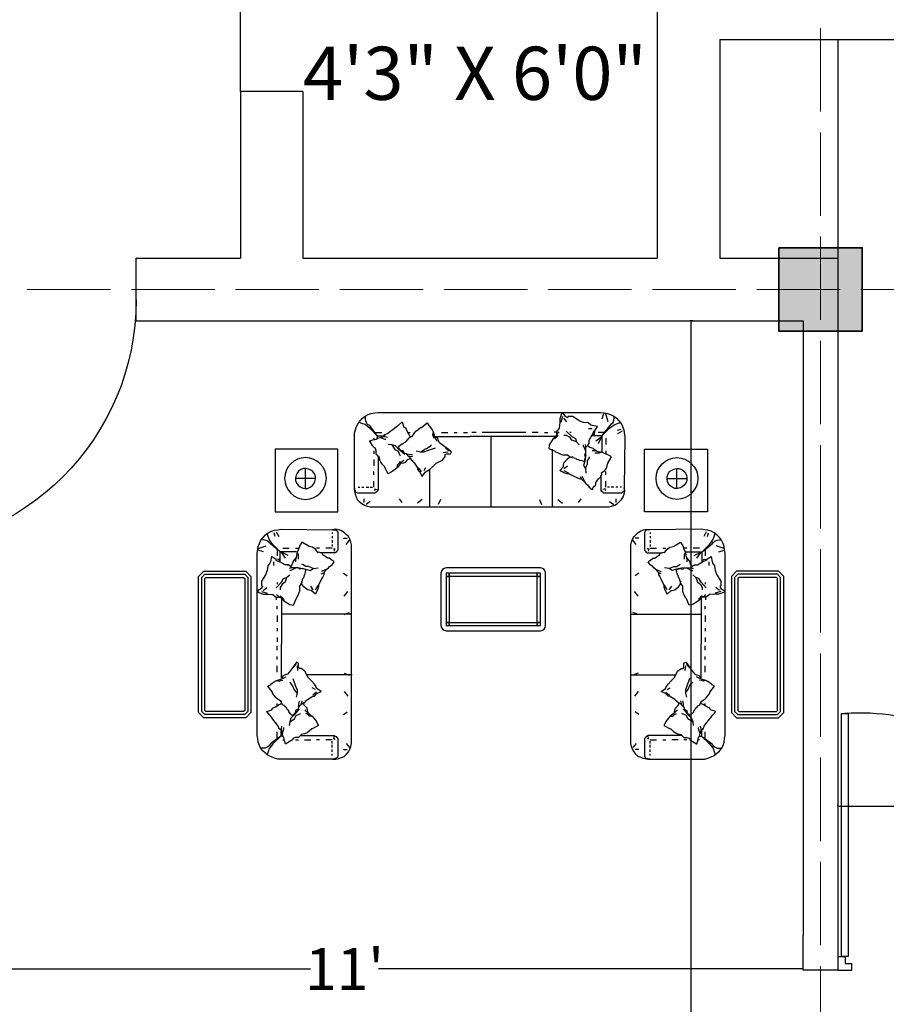
# Model space of a CAD drawing. Units: inches. Extents: x -113 to 5399, y -1393 to 3302.
# Tile 34 of 40: x 3405 to 3530, y 2762 to 2903. Entities that reach past the tile are written whole.
import ezdxf

# ---------------------------------------------------------------- set-up
doc = ezdxf.new("R2010")
doc.units = ezdxf.units.IN
doc.header["$MEASUREMENT"] = 0
doc.linetypes.add('ACAD_ISO02W100', pattern=[15, 12, -3])
doc.layers.add('24', color=7, linetype='Continuous')
for name, color, linetype, lineweight in [('A-ANNO-DIMS', 254, 'Continuous', 18), ('A-AREA-IDEN', 4, 'Continuous', 18), ('A-COLS', 7, 'Continuous', 35), ('doors', 2, 'Continuous', 25), ('furniture', 131, 'Continuous', 18), ('GRIDS', 7, 'ACAD_ISO02W100', 13), ('walls', 1, 'Continuous', 25)]:
    doc.layers.add(name, color=color, linetype=linetype, lineweight=lineweight)
doc.styles.get("Standard").update_dxf_attribs({"font": 'arial.ttf'})
doc.dimstyles.get("Standard").update_dxf_attribs({"dimtxt": 6, "dimasz": 0.18, "dimexe": 0.18, "dimexo": 0.0625, "dimgap": 0.09, "dimtad": 0, "dimtih": 1, "dimtoh": 1, "dimdec": 1, "dimzin": 0, "dimdsep": 46, "dimlunit": 4, "dimtxsty": 'Standard', "dimblk": 'ARCHTICK', "dimcen": 0.09, "dimadec": 0, "dimazin": 0, "dimtfac": 1, "dimtdec": 1, "dimtofl": 0, "dimtmove": 0, "dimatfit": 3, "dimfxl": 1, "dimtolj": 1, "dimtzin": 0, "dimarcsym": 0})

# ---------------------------------------------------------------- blocks, each defined once
blk = doc.blocks.new('*U3')
for p, q in [((0, 0), (0, -6)), ((36, 0), (36, -6))]:
    blk.add_line(p, q)
blk.add_lwpolyline([(0, 0), (0, 36), (1.75, 36), (1.75, 0)], close=True)
blk.add_arc((0, 0), 36, 0, 90)
blk = doc.blocks.new('DL13712')
at = {"layer": '24'}
for p, q in [((33, 28.5), (-34, 28.5)), ((33.5, -29.5), (-10, -29.5))]:
    blk.add_line(p, q, dxfattribs=at)
blk = doc.blocks.new('DL13976')
at = {"layer": '24'}
for p, q in [((-7, 18.5), (-3.5, 19.5)), ((-3.5, 19.5), (0.5, 20)), ((0.5, 20), (4.5, 19.5)), ((4.5, 19.5), (8, 18.5)), ((-18, 7.5), (-16, 11)), ((-16, 11), (-13.5, 14)), ((-13.5, 14), (-10.5, 16.5)), ((-10.5, 16.5), (-7, 18.5)), ((-2.5, 9), (0, 9.5)), ((0, 9.5), (2.5, 9.5)), ((0.5, -9.5), (0.5, 9.5)), ((2.5, 9.5), (5, 8.5)), ((8, 18.5), (11.5, 16.5)), ((11.5, 16.5), (14.5, 14)), ((14.5, 14), (17, 11)), ((17, 11), (19, 7.5)), ((-19.5, 0), (-19, 4)), ((-19, -4), (-19.5, 0)), ((-19, 4), (-18, 7.5)), ((-9, 2), (-8, 4.5)), ((-9, -0.5), (-9, 2)), ((-9, 0), (10, 0)), ((-8, 4.5), (-6.5, 6.5)), ((-6.5, 6.5), (-4.5, 8)), ((-5.5, 0), (6.5, 0)), ((-4.5, 8), (-2.5, 9)), ((0.5, -6), (0.5, 6)), ((5, 8.5), (7, 7)), ((7, 7), (8.5, 5)), ((8.5, 5), (9.5, 3)), ((9.5, 3), (10, 0.5)), ((10, 0.5), (10, -2)), ((19, 7.5), (20, 4)), ((20, 4), (20.5, 0)), ((20.5, 0), (20, -4)), ((-18, -7.5), (-19, -4)), ((-16, -11), (-18, -7.5)), ((-8.5, -3), (-9, -0.5)), ((-7.5, -5), (-8.5, -3)), ((-6, -7), (-7.5, -5)), ((-4, -8.5), (-6, -7)), ((-1.5, -9.5), (-4, -8.5)), ((3.5, -9), (1, -9.5)), ((5.5, -8), (3.5, -9)), ((7.5, -6.5), (5.5, -8)), ((9, -4.5), (7.5, -6.5)), ((10, -2), (9, -4.5)), ((19, -7.5), (17, -11)), ((20, -4), (19, -7.5)), ((-13.5, -14), (-16, -11)), ((-10.5, -16.5), (-13.5, -14)), ((-7, -18.5), (-10.5, -16.5)), ((-3.5, -19.5), (-7, -18.5)), ((1, -9.5), (-1.5, -9.5)), ((8, -18.5), (4.5, -19.5)), ((11.5, -16.5), (8, -18.5)), ((14.5, -14), (11.5, -16.5)), ((17, -11), (14.5, -14)), ((0.5, -20), (-3.5, -19.5)), ((4.5, -19.5), (0.5, -20))]:
    blk.add_line(p, q, dxfattribs=at)
blk = doc.blocks.new('DL13329')
at = {"layer": '24'}
for p, q in [((0, 0), (0, -60)), ((60, 0), (0, 0)), ((60, -60), (60, 0)), ((0, -60), (60, -60))]:
    blk.add_line(p, q, dxfattribs=at)
blk = doc.blocks.new('DL13303')
at = {"layer": '24'}
for p, q in [((-70, 20), (-65, 25)), ((-70, -20), (-70, 20)), ((-67, 19), (-64, 22)), ((-67, -19), (-67, 19)), ((-65, 25), (65, 25)), ((-64, 22), (64, 22)), ((-64, 18), (-63, 19)), ((-63, 19), (63, 19)), ((63, 19), (64, 18)), ((64, 22), (67, 19)), ((65, 25), (70, 20)), ((67, 19), (67, -19)), ((70, 20), (70, -20)), ((-64, -18), (-64, 18)), ((64, 18), (64, -18)), ((-63, -19), (-64, -18)), ((64, -18), (63, -19)), ((-65, -25), (-70, -20)), ((-64, -22), (-67, -19)), ((65, -25), (-65, -25)), ((64, -22), (-64, -22)), ((63, -19), (-63, -19)), ((67, -19), (64, -22)), ((70, -20), (65, -25))]:
    blk.add_line(p, q, dxfattribs=at)
blk = doc.blocks.new('DL12701')
at = {"layer": '24'}
for p, q in [((-104, 37.5), (-102, 40)), ((-102, 40), (-99.5, 42)), ((-99.5, 42), (-96.5, 43.5)), ((-99, 40), (-99, 42)), ((-99, 38), (-99, 40)), ((-98, 36), (-99, 38)), ((-96.5, 43.5), (-93.5, 44.5)), ((-93.5, 44.5), (-90, 45)), ((-90, 45), (-87, 45.5)), ((-87, 45.5), (0, 45.5)), ((0, 45.5), (87, 45.5)), ((50, 45), (48, 39.5)), ((48, 39.5), (48, 35.5)), ((50.5, 41.5), (49, 36)), ((51.5, 44.5), (50, 45)), ((53.5, 41.5), (51.5, 44.5)), ((51.5, 40), (54.5, 36.5)), ((55.5, 40.5), (53.5, 41.5)), ((56, 41.5), (55.5, 40.5)), ((60.5, 41.5), (56, 41.5)), ((66.5, 37.5), (60.5, 41.5)), ((87, 45.5), (90.5, 45)), ((88.5, 39.5), (90, 44.5)), ((90.5, 45), (93.5, 44.5)), ((91.5, 44.5), (94, 37)), ((93.5, 44.5), (96.5, 43.5)), ((96.5, 43.5), (99.5, 42)), ((99, 36), (99.5, 38)), ((99.5, 42), (102, 40)), ((100, 40), (99.5, 42)), ((99.5, 38), (100, 40)), ((102, 40), (104.5, 37.5)), ((-109.5, 26), (-108.5, 29)), ((-108.5, 29), (-107.5, 32)), ((-107.5, 32), (-106, 35)), ((-106, 35), (-104, 37.5)), ((-102.5, 35), (-105, 36)), ((-99.5, 34), (-102.5, 35)), ((-97, 32), (-99.5, 34)), ((-97, 34), (-98, 36)), ((-95, 33), (-97, 34)), ((-95, 30.5), (-97, 32)), ((-87.5, 23), (-95, 33)), ((-87.5, 23), (-95, 30.5)), ((-76, 27), (-71.5, 30.5)), ((-71.5, 30.5), (-69.5, 32)), ((-69.5, 32), (-67.5, 33.5)), ((-67.5, 33.5), (-64, 36.5)), ((-64, 36.5), (-62.5, 31.5)), ((-62.5, 31.5), (-61, 31)), ((-61, 31), (-59.5, 28)), ((-51, 27.5), (-49, 29)), ((-49, 29), (-46.5, 31)), ((-46.5, 31), (-45.5, 31)), ((-45.5, 31), (-40, 35.5)), ((-40, 35.5), (-38.5, 33)), ((-38.5, 33), (-38, 32.5)), ((-38, 32.5), (-35.5, 29)), ((-35.5, 29), (-34.5, 27)), ((47.5, 30.5), (45.5, 28)), ((48, 35.5), (47.5, 30.5)), ((70.5, 36), (66.5, 37.5)), ((75, 35.5), (70.5, 36)), ((77.5, 33.5), (75, 35.5)), ((79, 30), (75.5, 30)), ((79, 33), (77.5, 33.5)), ((84, 32), (79, 33)), ((81.5, 28), (84, 32)), ((88.5, 23.5), (96, 33)), ((88.5, 23.5), (95.5, 30.5)), ((95.5, 30.5), (98, 32.5)), ((96, 33), (97.5, 34.5)), ((97.5, 34.5), (99, 36)), ((98, 32.5), (100.5, 34)), ((100.5, 34), (103, 35)), ((103, 35), (106, 36)), ((103, 28.5), (106.5, 29.5)), ((104.5, 37.5), (106.5, 35)), ((106.5, 35), (108, 32)), ((108, 32), (109, 29)), ((109, 29), (109.5, 26)), ((-109.5, 22.5), (-109.5, 26)), ((-109.5, -26.5), (-109.5, 22.5)), ((-95, 18.5), (-92, 19.5)), ((-92, 19.5), (-89, 20)), ((-91, 21), (-91, 19.5)), ((-89.5, 26.5), (-83.5, 26.5)), ((-89, 20), (-87.5, 21)), ((-87.5, 21), (-87.5, 23)), ((-81.5, 23), (-87.5, 23)), ((-87.5, 21), (-85, 21.5)), ((-85, 21.5), (-82, 22.5)), ((-85, 21.5), (-80.5, 20)), ((-82, 22.5), (-80.5, 24.5)), ((-82, 22.5), (-80.5, 22.5)), ((-80.5, 24.5), (-78, 25.5)), ((-80.5, 24.5), (-80.5, 23.5)), ((-80.5, 22.5), (-78, 22)), ((-80.5, 20), (-79.5, 20)), ((-78, 25.5), (-76, 27)), ((-77, 25.5), (-77, 25.5)), ((-60.5, 17.5), (-59, 19.5)), ((-59.5, 28), (-57.5, 24.5)), ((-59, 19.5), (-58.5, 19.5)), ((-58.5, 19.5), (-58, 21)), ((-58, 26.5), (-56.5, 26.5)), ((-58, 21), (-54.5, 23)), ((-57.5, 24.5), (-56.5, 22)), ((-56.5, 22.5), (-54.5, 22.5)), ((-54.5, 22.5), (-52.5, 25.5)), ((-54.5, 23), (-54.5, 22.5)), ((-54, 22.5), (-54, 22.5)), ((-52.5, 25.5), (-52, 26.5)), ((-52, 26.5), (-51, 27.5)), ((-34.5, 27), (-35, 24.5)), ((-35, 24.5), (-34.5, 23)), ((-34.5, 27), (-33.5, 24)), ((-34.5, 23), (-34, 21)), ((-33.5, 24), (-33, 22)), ((-30, 21), (-33, 22)), ((-33, 22), (-31.5, 19.5)), ((-32, 22.5), (0.5, 22.5)), ((-31.5, 19.5), (-31, 18)), ((-29.5, 19.5), (-30, 21)), ((-28.5, 16.5), (-29.5, 19.5)), ((-26.5, 26.5), (-20.5, 26.5)), ((-14.5, 26.5), (-11.5, 26.5)), ((-5.5, 26.5), (-1.5, 26.5)), ((44, 22.5), (0.5, 22.5)), ((6.5, 26.5), (2.5, 26.5)), ((15.5, 26.5), (12.5, 26.5)), ((27.5, 26.5), (21.5, 26.5)), ((33.5, 26.5), (36.5, 26.5)), ((41.5, 20), (40.5, 18.5)), ((43.5, 22), (41.5, 20)), ((43.5, 20.5), (41.5, 20)), ((42.5, 27), (45, 27)), ((45, 23.5), (43.5, 22)), ((45, 22), (43.5, 20.5)), ((45.5, 28), (45, 27)), ((45, 27), (45, 23.5)), ((45, 23.5), (46.5, 26)), ((46.5, 23.5), (45, 22)), ((46.5, 26), (47.5, 27)), ((54.5, 23.5), (52, 23.5)), ((54, 27.5), (59.5, 22.5)), ((58, 21.5), (54.5, 23.5)), ((59, 26.5), (57.5, 26.5)), ((59.5, 19), (58, 21.5)), ((59.5, 22.5), (63, 20.5)), ((64, 17.5), (59.5, 19)), ((63, 20.5), (64, 17.5)), ((76, 19), (79, 24)), ((76, 16), (76, 19)), ((80.5, 28), (79, 24)), ((79, 24), (81, 24.5)), ((79, 23.5), (88.5, 23.5)), ((81, 24.5), (81.5, 28)), ((82.5, 18.5), (88, 22.5)), ((90.5, 26.5), (84.5, 26.5)), ((85, 16), (88, 22.5)), ((88.5, 8), (88.5, 23.5)), ((92, 21), (92, 15)), ((107.5, 27.5), (103, 25)), ((109.5, 26), (110, 22.5)), ((110, 22.5), (109.5, -26.5)), ((-95, 18), (-95, 18.5)), ((-94, 16.5), (-95, 18)), ((-92.5, 14), (-94, 16.5)), ((-92, 13.5), (-92.5, 14)), ((-91.5, 12.5), (-92, 13.5)), ((-89.5, 11), (-91.5, 12.5)), ((-89, 9), (-89.5, 11)), ((-74, 14.5), (-77.5, 15)), ((-70.5, 13.5), (-74, 14.5)), ((-74, 14.5), (-71, 10)), ((-71, 10), (-68, 8.5)), ((-67.5, 10.5), (-70.5, 13.5)), ((-68, 12), (-67.5, 12.5)), ((-65, 9), (-68, 12)), ((-67.5, 12.5), (-66.5, 13.5)), ((-61.5, 5.5), (-67.5, 10.5)), ((-66.5, 13.5), (-64.5, 15.5)), ((-64.5, 15.5), (-63.5, 15.5)), ((-63.5, 15.5), (-62.5, 16.5)), ((-62.5, 16.5), (-60.5, 17.5)), ((-46.5, 7.5), (-42.5, 10.5)), ((-42.5, 10.5), (-40, 11.5)), ((-40, 11.5), (-37, 13.5)), ((-32.5, 11.5), (-40, 9)), ((-37, 13.5), (-36, 14.5)), ((-24.5, 13.5), (-28.5, 16.5)), ((-21, 11), (-24.5, 13.5)), ((-19, 8.5), (-22.5, 11.5)), ((-17, 8), (-21, 11)), ((38, 14), (37.5, 11)), ((37.5, 11), (43.5, 8.5)), ((40.5, 18.5), (38, 14.5)), ((38, 14.5), (38, 14)), ((64, 17.5), (66.5, 14.5)), ((70.5, 13.5), (70.5, 14.5)), ((73, 8.5), (70.5, 13.5)), ((73, 13), (72.5, 15)), ((73, 12.5), (75, 14.5)), ((73, 12.5), (73, 13)), ((73, 8.5), (73, 12.5)), ((76, 12.5), (74, 14)), ((75, 14.5), (76, 16)), ((75.5, 16), (76, 16.5)), ((80, 11), (76, 12.5)), ((80.5, 10.5), (80, 11)), ((83, 8.5), (80.5, 10.5)), ((-91, 9), (-91, 6)), ((-91, 0.5), (-91, -5.5)), ((-89, 8.5), (-89, 9)), ((-89, 6), (-89, 8.5)), ((-86.5, 3.5), (-89, 6)), ((-87, 3.5), (-87, -26.5)), ((-86, 3.5), (-86.5, 3.5)), ((-85.5, 0.5), (-86, 3.5)), ((-85.5, 0), (-85.5, 0.5)), ((-84.5, -2), (-85.5, 0)), ((-68, 8.5), (-66.5, 5.5)), ((-66.5, 5.5), (-66, 4)), ((-63, 9), (-65, 9)), ((-62.5, 0), (-63.5, -1)), ((-62, 6.5), (-63, 9)), ((-60, 6), (-62, 6.5)), ((-61, -2), (-58.5, 0.5)), ((-57.5, 3.5), (-60, 6)), ((-60, 6), (-55, 5.5)), ((-58.5, 0.5), (-55.5, 2)), ((-56.5, 3.5), (-57.5, 3.5)), ((-57.5, 3.5), (-56, 1.5)), ((-54, 3), (-56.5, 3.5)), ((-56, 1.5), (-55, 0)), ((-55, 5.5), (-54, 5)), ((-55, 0), (-52.5, -2.5)), ((-46.5, 7.5), (-50.5, 8.5)), ((-43.5, 7.5), (-46.5, 7.5)), ((-40, 9), (-43.5, 7.5)), ((-31.5, -3), (-25.5, 0)), ((-25.5, 0), (-23, 3.5)), ((-20.5, 7.5), (-25, 7)), ((-23, 5.5), (-21.5, 6)), ((-23, 3.5), (-23, 5.5)), ((-21.5, 6), (-18, 6)), ((-18, 6), (-17, 8)), ((43.5, 8.5), (44, 8)), ((44, 8), (47, 6.5)), ((47, 6.5), (49.5, 5.5)), ((49.5, 5.5), (51, 5)), ((51, 5), (52.5, 5)), ((52, -2.5), (55, 1)), ((52.5, 5), (55.5, 5)), ((55, 1), (57.5, 3)), ((55.5, 5), (55.5, 5)), ((55.5, 5), (59, 2.5)), ((59, 2.5), (60, 3.5)), ((60, 3.5), (60, 2.5)), ((60, 2.5), (63, 2)), ((63, 2), (64, 1)), ((64, 1), (66, 0.5)), ((66, 0.5), (66.5, 0)), ((66.5, 0), (69, -0.5)), ((71.5, -1), (72.5, 2.5)), ((72, 5), (73, 6.5)), ((73, 5.5), (72, -1)), ((72.5, 2.5), (72, 5)), ((73, 6.5), (73, 8.5)), ((74.5, -0.5), (76, 1.5)), ((76, 1.5), (76.5, 3)), ((80.5, 9), (79, 9)), ((83, 8.5), (80.5, 9)), ((84, 6.5), (81.5, 6.5)), ((85, 8), (83, 8.5)), ((85.5, 6.5), (84, 6.5)), ((88, 7.5), (85, 8)), ((88, 7.5), (85.5, 6.5)), ((90, 6.5), (88, 7.5)), ((94, 5), (90, 6.5)), ((92, 9), (92, 6)), ((95, 4.5), (94, 5)), ((94, -3), (97.5, 3)), ((97.5, 3), (95, 4.5)), ((-83, -4), (-84.5, -2)), ((-80.5, -6.5), (-83, -4)), ((-80.5, -7), (-80.5, -6.5)), ((-77.5, -13), (-80.5, -7)), ((-70.5, -8.5), (-73.5, -11)), ((-68.5, -7), (-70.5, -8.5)), ((-68.5, -4.5), (-67, -3)), ((-66.5, -4.5), (-68.5, -7)), ((-68.5, -7), (-68.5, -4.5)), ((-67, -3), (-66, -1)), ((-65.5, -3), (-66.5, -4.5)), ((-63.5, -1), (-65.5, -3)), ((-65.5, -3), (-62.5, -2.5)), ((-62.5, -2.5), (-61, -2)), ((-54, -0.5), (-53.5, -0.5)), ((-52.5, -2.5), (-49.5, -7.5)), ((-49.5, -7.5), (-49.5, -9)), ((-49.5, -9), (-47, -11.5)), ((-45.5, -11), (-48.5, -7.5)), ((-43, -10), (-41.5, -7)), ((-41, -11), (-38, -9)), ((-38, -9), (-35, -6.5)), ((-35, -6.5), (-31.5, -3)), ((48, -10), (51.5, -6)), ((51.5, -5.5), (52, -2.5)), ((51.5, -6), (51.5, -5.5)), ((52, -8), (55.5, -5.5)), ((69, -0.5), (70.5, -1)), ((70.5, -1), (71.5, -1)), ((72, -1), (70.5, -5)), ((70.5, -5), (72.5, -8)), ((72.5, -8), (74.5, -3.5)), ((72.5, -8), (73, -12.5)), ((74.5, -3.5), (74.5, -0.5)), ((91, -10), (92, -8.5)), ((92, -8.5), (93, -7)), ((93, -7), (93.5, -4)), ((93.5, -4), (94, -3)), ((-91, -14), (-91, -11)), ((-74.5, -11.5), (-77.5, -13)), ((-73.5, -11), (-74.5, -11.5)), ((-47, -11.5), (-45, -15.5)), ((-45, -15.5), (-42, -11.5)), ((-42, -11.5), (-41, -11)), ((52, -12), (48, -10)), ((52, -10), (56.5, -12.5)), ((55, -13), (52, -12)), ((56.5, -13), (55, -13)), ((62.5, -16), (56.5, -13)), ((64.5, -17), (62.5, -16)), ((64, -16.5), (64, -16.5)), ((66.5, -18), (64.5, -17)), ((69, -18.5), (66.5, -18)), ((67.5, -15.5), (68.5, -18)), ((68.5, -18), (69, -18.5)), ((69, -18.5), (72, -21)), ((70, -16.5), (69.5, -15.5)), ((72, -21), (70, -16.5)), ((83.5, -20), (85, -18)), ((85, -17.5), (87, -16.5)), ((85, -18), (85, -17.5)), ((87, -16.5), (88, -13)), ((87.5, -12.5), (89.5, -11)), ((88, -13), (87.5, -12.5)), ((87.5, -26.5), (87.5, -14.5)), ((89.5, -11), (91, -10)), ((92, -14), (92, -11)), ((-109.5, -28), (-109.5, -26.5)), ((-109.5, -26.5), (-109.5, -29.5)), ((-109, -29), (-109.5, -28)), ((-106, -26), (-104.5, -26)), ((-102.5, -26), (-100.5, -26)), ((-98.5, -26), (-96, -26)), ((-94.5, -26), (-92.5, -26)), ((-91, -26), (-91, -20)), ((-90.5, -27.5), (-88, -28)), ((-90.5, -28), (-90, -29)), ((-87, -28), (-87.5, -29)), ((-87, -26.5), (-87, -28)), ((72, -21), (73, -22.5)), ((73, -22.5), (74.5, -23.5)), ((74.5, -23.5), (76, -26)), ((76, -26), (79, -28)), ((79, -28), (79.5, -27.5)), ((79.5, -27.5), (80, -26)), ((80, -26), (82.5, -23.5)), ((82.5, -21.5), (83.5, -20)), ((82.5, -22.5), (82.5, -21.5)), ((82.5, -23.5), (82.5, -22.5)), ((87.5, -28), (87.5, -26.5)), ((87.5, -29), (87.5, -28)), ((91.5, -27.5), (89, -28)), ((91.5, -28), (91, -29)), ((92, -26), (92, -20)), ((95.5, -26), (93.5, -26)), ((99.5, -26), (97, -26)), ((103.5, -26), (101.5, -26)), ((107, -26), (105.5, -26)), ((110, -29.5), (109.5, -26.5)), ((109.5, -26.5), (109.5, -28)), ((109.5, -28), (109.5, -29)), ((-109.5, -29.5), (-109, -32.5)), ((-108.5, -30), (-109, -29)), ((-109, -32.5), (-108, -35)), ((-108, -31), (-108.5, -30)), ((-106.5, -31.5), (-108, -31)), ((-108, -35), (-107, -37.5)), ((-107, -37.5), (-105, -39.5)), ((-105.5, -31.5), (-106.5, -31.5)), ((-104.5, -31.5), (-105.5, -31.5)), ((-92, -31.5), (-104.5, -31.5)), ((-100.5, -37), (-100.5, -40.5)), ((-91, -31.5), (-92, -31.5)), ((-90, -31.5), (-91, -31.5)), ((-89, -30.5), (-90, -31.5)), ((-88, -30), (-89, -30.5)), ((-87.5, -29), (-88, -30)), ((-67, -37), (-64.5, -40.5)), ((-45, -37.5), (-49.5, -41)), ((-27.5, -37.5), (-29.5, -42.5)), ((28.5, -37.5), (30.5, -42.5)), ((46, -37.5), (50.5, -41)), ((68, -37), (65.5, -40.5)), ((88, -30), (87.5, -29)), ((89, -30.5), (88, -30)), ((90, -31.5), (89, -30.5)), ((91, -31.5), (90, -31.5)), ((92.5, -31.5), (91, -31.5)), ((104.5, -31.5), (92.5, -31.5)), ((101.5, -37), (101.5, -40.5)), ((106, -31.5), (104.5, -31.5)), ((105, -39.5), (107, -37.5)), ((107, -31.5), (106, -31.5)), ((108, -31), (107, -31.5)), ((107, -37.5), (108.5, -35)), ((109, -30), (108, -31)), ((108.5, -35), (109.5, -32.5)), ((109.5, -29), (109, -30)), ((109.5, -32.5), (110, -29.5)), ((-105, -39.5), (-102.5, -41.5)), ((-102.5, -41.5), (-100, -43)), ((-100, -43), (-97.5, -44)), ((-94.5, -39.5), (-98.5, -42.5)), ((-97.5, -44), (-94.5, -44.5)), ((-94.5, -44.5), (0, -44.5)), ((0, -44.5), (95, -44.5)), ((95, -44.5), (97.5, -44)), ((95.5, -39.5), (99.5, -42.5)), ((97.5, -44), (100.5, -43)), ((100.5, -43), (103, -41.5)), ((103, -41.5), (105, -39.5))]:
    blk.add_line(p, q, dxfattribs=at)
blk = doc.blocks.new('DL13707')
at = {"layer": '24'}
for p, q in [((0, -33.5), (0, 33.5)), ((-58.5, -33.5), (-58.5, 21.5)), ((58.5, -33.5), (58.5, 2))]:
    blk.add_line(p, q, dxfattribs=at)
blk = doc.blocks.new('DL13651')
at = {"layer": '24'}
for p, q in [((-50, 27), (-49, 28.5)), ((-49, 28.5), (-47.5, 29.5)), ((-47.5, 29.5), (-45.5, 30)), ((-45.5, 30), (44.5, 30)), ((44.5, 30), (46.5, 29.5)), ((46.5, 29.5), (48, 28.5)), ((48, 28.5), (49, 27)), ((-50.5, 25), (-50, 27)), ((-50.5, -25), (-50.5, 25)), ((-45.5, 24.5), (-45.5, 25)), ((-45.5, 25), (-45, 25)), ((-45.5, -24.5), (-45.5, 24.5)), ((-45, 25), (44, 25)), ((-45, 22), (44, 22)), ((-42.5, 22), (-45, 22)), ((-42.5, -24.5), (-42.5, 24.5)), ((-42.5, 24.5), (-42.5, 22)), ((41.5, 22), (41.5, 24.5)), ((41.5, 24.5), (41.5, -24.5)), ((44, 22), (41.5, 22)), ((44, 25), (44.5, 25)), ((44.5, 25), (44.5, 24.5)), ((44.5, 24.5), (44.5, -24.5)), ((49, 27), (49.5, 25)), ((49.5, 25), (49.5, -25)), ((-50, -27), (-50.5, -25)), ((-49, -28.5), (-50, -27)), ((-45.5, -25), (-45.5, -24.5)), ((-45, -25), (-45.5, -25)), ((44, -22), (-45, -22)), ((-45, -22), (-42.5, -22)), ((44, -25), (-45, -25)), ((-42.5, -22), (-42.5, -24.5)), ((41.5, -24.5), (41.5, -22)), ((41.5, -22), (44, -22)), ((44.5, -25), (44, -25)), ((44.5, -24.5), (44.5, -25)), ((49, -27), (48, -28.5)), ((49.5, -25), (49, -27)), ((-47.5, -29.5), (-49, -28.5)), ((-45.5, -30), (-47.5, -29.5)), ((44.5, -30), (-45.5, -30)), ((46.5, -29.5), (44.5, -30)), ((48, -28.5), (46.5, -29.5))]:
    blk.add_line(p, q, dxfattribs=at)
blk = doc.blocks.new('DL12263')
at = {"layer": '24'}
for p, q in [((-123, 37.5), (-121, 40)), ((-121, 40), (-118.5, 42)), ((-118.5, 42), (-115.5, 43.5)), ((-118, 40), (-118, 42)), ((-118, 38), (-118, 40)), ((-117, 36), (-118, 38)), ((-115.5, 43.5), (-112.5, 44.5)), ((-112.5, 44.5), (-109, 45)), ((-109, 45), (-106, 45.5)), ((-106, 45.5), (-19, 45.5)), ((-19, 45.5), (106.5, 45.5)), ((69.5, 45), (67.5, 39.5)), ((67.5, 39.5), (67.5, 35.5)), ((70, 41.5), (68.5, 36)), ((71, 44.5), (69.5, 45)), ((73, 41.5), (71, 44.5)), ((71, 40), (74, 36.5)), ((75, 40.5), (73, 41.5)), ((75.5, 41.5), (75, 40.5)), ((80, 41.5), (75.5, 41.5)), ((86, 37.5), (80, 41.5)), ((106.5, 45.5), (110, 45)), ((108, 39.5), (109.5, 44.5)), ((110, 45), (113, 44.5)), ((111, 44.5), (113.5, 37)), ((113, 44.5), (116, 43.5)), ((116, 43.5), (119, 42)), ((118.5, 36), (119, 38)), ((119, 42), (121.5, 40)), ((119.5, 40), (119, 42)), ((119, 38), (119.5, 40)), ((121.5, 40), (124, 37.5)), ((-128.5, 26), (-127.5, 29)), ((-127.5, 29), (-126.5, 32)), ((-126.5, 32), (-125, 35)), ((-125, 35), (-123, 37.5)), ((-121.5, 35), (-124, 36)), ((-118.5, 34), (-121.5, 35)), ((-116, 32), (-118.5, 34)), ((-116, 34), (-117, 36)), ((-114, 33), (-116, 34)), ((-114, 30.5), (-116, 32)), ((-106.5, 23), (-114, 33)), ((-106.5, 23), (-114, 30.5)), ((-95, 27), (-90.5, 30.5)), ((-90.5, 30.5), (-88.5, 32)), ((-88.5, 32), (-86.5, 33.5)), ((-86.5, 33.5), (-83, 36.5)), ((-83, 36.5), (-81.5, 31.5)), ((-81.5, 31.5), (-80, 31)), ((-80, 31), (-78.5, 28)), ((-70, 27.5), (-68, 29)), ((-68, 29), (-65.5, 31)), ((-65.5, 31), (-64.5, 31)), ((-64.5, 31), (-59, 35.5)), ((-59, 35.5), (-57.5, 33)), ((-57.5, 33), (-57, 32.5)), ((-57, 32.5), (-54.5, 29)), ((-54.5, 29), (-53.5, 27)), ((67, 30.5), (65, 28)), ((67.5, 35.5), (67, 30.5)), ((90, 36), (86, 37.5)), ((94.5, 35.5), (90, 36)), ((97, 33.5), (94.5, 35.5)), ((98.5, 30), (95, 30)), ((98.5, 33), (97, 33.5)), ((103.5, 32), (98.5, 33)), ((101, 28), (103.5, 32)), ((108, 23.5), (115.5, 33)), ((108, 23.5), (115, 30.5)), ((115, 30.5), (117.5, 32.5)), ((115.5, 33), (117, 34.5)), ((117, 34.5), (118.5, 36)), ((117.5, 32.5), (120, 34)), ((120, 34), (122.5, 35)), ((122.5, 35), (125.5, 36)), ((122.5, 28.5), (126, 29.5)), ((124, 37.5), (126, 35)), ((126, 35), (127.5, 32)), ((127.5, 32), (128.5, 29)), ((128.5, 29), (129, 26)), ((-128.5, 22.5), (-128.5, 26)), ((-128.5, -26.5), (-128.5, 22.5)), ((-114, 18.5), (-111, 19.5)), ((-111, 19.5), (-108, 20)), ((-110, 21), (-110, 19.5)), ((-108.5, 26.5), (-102.5, 26.5)), ((-108, 20), (-106.5, 21)), ((-106.5, 21), (-106.5, 23)), ((-100.5, 23), (-106.5, 23)), ((-106.5, 21), (-104, 21.5)), ((-104, 21.5), (-101, 22.5)), ((-104, 21.5), (-99.5, 20)), ((-101, 22.5), (-99.5, 24.5)), ((-101, 22.5), (-99.5, 22.5)), ((-99.5, 24.5), (-97, 25.5)), ((-99.5, 24.5), (-99.5, 23.5)), ((-99.5, 22.5), (-97, 22)), ((-99.5, 20), (-98.5, 20)), ((-97, 25.5), (-95, 27)), ((-96, 25.5), (-96, 25.5)), ((-79.5, 17.5), (-78, 19.5)), ((-78.5, 28), (-76.5, 24.5)), ((-78, 19.5), (-77.5, 19.5)), ((-77.5, 19.5), (-77, 21)), ((-77, 26.5), (-75.5, 26.5)), ((-77, 21), (-73.5, 23)), ((-76.5, 24.5), (-75.5, 22)), ((-75.5, 22.5), (-73.5, 22.5)), ((-73.5, 22.5), (-71.5, 25.5)), ((-73.5, 23), (-73.5, 22.5)), ((-73, 22.5), (-73, 22.5)), ((-71.5, 25.5), (-71, 26.5)), ((-71, 26.5), (-70, 27.5)), ((-53.5, 27), (-54, 24.5)), ((-54, 24.5), (-53.5, 23)), ((-53.5, 27), (-52.5, 24)), ((-53.5, 23), (-53, 21)), ((-52.5, 24), (-52, 22)), ((-49, 21), (-52, 22)), ((-52, 22), (-50.5, 19.5)), ((-51, 22.5), (-18.5, 22.5)), ((-50.5, 19.5), (-50, 18)), ((-48.5, 19.5), (-49, 21)), ((-47.5, 16.5), (-48.5, 19.5)), ((-45.5, 26.5), (-39.5, 26.5)), ((-33.5, 26.5), (-30.5, 26.5)), ((-24.5, 26.5), (-20.5, 26.5)), ((63.5, 22.5), (-18.5, 22.5)), ((-12.5, 26.5), (-16.5, 26.5)), ((35, 26.5), (-6.5, 26.5)), ((47, 26.5), (41, 26.5)), ((53, 26.5), (56, 26.5)), ((61, 20), (60, 18.5)), ((63, 22), (61, 20)), ((63, 20.5), (61, 20)), ((62, 27), (64.5, 27)), ((64.5, 23.5), (63, 22)), ((64.5, 22), (63, 20.5)), ((65, 28), (64.5, 27)), ((64.5, 27), (64.5, 23.5)), ((64.5, 23.5), (66, 26)), ((66, 23.5), (64.5, 22)), ((66, 26), (67, 27)), ((74, 23.5), (71.5, 23.5)), ((73.5, 27.5), (79, 22.5)), ((77.5, 21.5), (74, 23.5)), ((78.5, 26.5), (77, 26.5)), ((79, 19), (77.5, 21.5)), ((79, 22.5), (82.5, 20.5)), ((83.5, 17.5), (79, 19)), ((82.5, 20.5), (83.5, 17.5)), ((95.5, 19), (98.5, 24)), ((95.5, 16), (95.5, 19)), ((100, 28), (98.5, 24)), ((98.5, 24), (100.5, 24.5)), ((98.5, 23.5), (108, 23.5)), ((100.5, 24.5), (101, 28)), ((102, 18.5), (107.5, 22.5)), ((110, 26.5), (104, 26.5)), ((104.5, 16), (107.5, 22.5)), ((108, 8), (108, 23.5)), ((111.5, 21), (111.5, 15)), ((127, 27.5), (122.5, 25)), ((129, 26), (129.5, 22.5)), ((129.5, 22.5), (129, -26.5)), ((-114, 18), (-114, 18.5)), ((-113, 16.5), (-114, 18)), ((-111.5, 14), (-113, 16.5)), ((-111, 13.5), (-111.5, 14)), ((-110.5, 12.5), (-111, 13.5)), ((-108.5, 11), (-110.5, 12.5)), ((-108, 9), (-108.5, 11)), ((-93, 14.5), (-96.5, 15)), ((-89.5, 13.5), (-93, 14.5)), ((-93, 14.5), (-90, 10)), ((-90, 10), (-87, 8.5)), ((-86.5, 10.5), (-89.5, 13.5)), ((-87, 12), (-86.5, 12.5)), ((-84, 9), (-87, 12)), ((-86.5, 12.5), (-85.5, 13.5)), ((-80.5, 5.5), (-86.5, 10.5)), ((-85.5, 13.5), (-83.5, 15.5)), ((-83.5, 15.5), (-82.5, 15.5)), ((-82.5, 15.5), (-81.5, 16.5)), ((-81.5, 16.5), (-79.5, 17.5)), ((-65.5, 7.5), (-61.5, 10.5)), ((-61.5, 10.5), (-59, 11.5)), ((-59, 11.5), (-56, 13.5)), ((-51.5, 11.5), (-59, 9)), ((-56, 13.5), (-55, 14.5)), ((-43.5, 13.5), (-47.5, 16.5)), ((-40, 11), (-43.5, 13.5)), ((-38, 8.5), (-41.5, 11.5)), ((-36, 8), (-40, 11)), ((57.5, 14), (57, 11)), ((57, 11), (63, 8.5)), ((60, 18.5), (57.5, 14.5)), ((57.5, 14.5), (57.5, 14)), ((83.5, 17.5), (86, 14.5)), ((90, 13.5), (90, 14.5)), ((92.5, 8.5), (90, 13.5)), ((92.5, 13), (92, 15)), ((92.5, 12.5), (94.5, 14.5)), ((92.5, 12.5), (92.5, 13)), ((92.5, 8.5), (92.5, 12.5)), ((95.5, 12.5), (93.5, 14)), ((94.5, 14.5), (95.5, 16)), ((95, 16), (95.5, 16.5)), ((99.5, 11), (95.5, 12.5)), ((100, 10.5), (99.5, 11)), ((102.5, 8.5), (100, 10.5)), ((-110, 9), (-110, 6)), ((-110, 0.5), (-110, -5.5)), ((-108, 8.5), (-108, 9)), ((-108, 6), (-108, 8.5)), ((-105.5, 3.5), (-108, 6)), ((-106, 3.5), (-106, -26.5)), ((-105, 3.5), (-105.5, 3.5)), ((-104.5, 0.5), (-105, 3.5)), ((-104.5, 0), (-104.5, 0.5)), ((-103.5, -2), (-104.5, 0)), ((-87, 8.5), (-85.5, 5.5)), ((-85.5, 5.5), (-85, 4)), ((-82, 9), (-84, 9)), ((-81.5, 0), (-82.5, -1)), ((-81, 6.5), (-82, 9)), ((-79, 6), (-81, 6.5)), ((-80, -2), (-77.5, 0.5)), ((-76.5, 3.5), (-79, 6)), ((-79, 6), (-74, 5.5)), ((-77.5, 0.5), (-74.5, 2)), ((-75.5, 3.5), (-76.5, 3.5)), ((-76.5, 3.5), (-75, 1.5)), ((-73, 3), (-75.5, 3.5)), ((-75, 1.5), (-74, 0)), ((-74, 5.5), (-73, 5)), ((-74, 0), (-71.5, -2.5)), ((-65.5, 7.5), (-69.5, 8.5)), ((-62.5, 7.5), (-65.5, 7.5)), ((-59, 9), (-62.5, 7.5)), ((-50.5, -3), (-44.5, 0)), ((-44.5, 0), (-42, 3.5)), ((-39.5, 7.5), (-44, 7)), ((-42, 5.5), (-40.5, 6)), ((-42, 3.5), (-42, 5.5)), ((-40.5, 6), (-37, 6)), ((-37, 6), (-36, 8)), ((63, 8.5), (63.5, 8)), ((63.5, 8), (66.5, 6.5)), ((66.5, 6.5), (69, 5.5)), ((69, 5.5), (70.5, 5)), ((70.5, 5), (72, 5)), ((71.5, -2.5), (74.5, 1)), ((72, 5), (75, 5)), ((74.5, 1), (77, 3)), ((75, 5), (75, 5)), ((75, 5), (78.5, 2.5)), ((78.5, 2.5), (79.5, 3.5)), ((79.5, 3.5), (79.5, 2.5)), ((79.5, 2.5), (82.5, 2)), ((82.5, 2), (83.5, 1)), ((83.5, 1), (85.5, 0.5)), ((85.5, 0.5), (86, 0)), ((86, 0), (88.5, -0.5)), ((91, -1), (92, 2.5)), ((91.5, 5), (92.5, 6.5)), ((92.5, 5.5), (91.5, -1)), ((92, 2.5), (91.5, 5)), ((92.5, 6.5), (92.5, 8.5)), ((94, -0.5), (95.5, 1.5)), ((95.5, 1.5), (96, 3)), ((100, 9), (98.5, 9)), ((102.5, 8.5), (100, 9)), ((103.5, 6.5), (101, 6.5)), ((104.5, 8), (102.5, 8.5)), ((105, 6.5), (103.5, 6.5)), ((107.5, 7.5), (104.5, 8)), ((107.5, 7.5), (105, 6.5)), ((109.5, 6.5), (107.5, 7.5)), ((113.5, 5), (109.5, 6.5)), ((111.5, 9), (111.5, 6)), ((114.5, 4.5), (113.5, 5)), ((113.5, -3), (117, 3)), ((117, 3), (114.5, 4.5)), ((-102, -4), (-103.5, -2)), ((-99.5, -6.5), (-102, -4)), ((-99.5, -7), (-99.5, -6.5)), ((-96.5, -13), (-99.5, -7)), ((-89.5, -8.5), (-92.5, -11)), ((-87.5, -7), (-89.5, -8.5)), ((-87.5, -4.5), (-86, -3)), ((-85.5, -4.5), (-87.5, -7)), ((-87.5, -7), (-87.5, -4.5)), ((-86, -3), (-85, -1)), ((-84.5, -3), (-85.5, -4.5)), ((-82.5, -1), (-84.5, -3)), ((-84.5, -3), (-81.5, -2.5)), ((-81.5, -2.5), (-80, -2)), ((-73, -0.5), (-72.5, -0.5)), ((-71.5, -2.5), (-68.5, -7.5)), ((-68.5, -7.5), (-68.5, -9)), ((-68.5, -9), (-66, -11.5)), ((-64.5, -11), (-67.5, -7.5)), ((-62, -10), (-60.5, -7)), ((-60, -11), (-57, -9)), ((-57, -9), (-54, -6.5)), ((-54, -6.5), (-50.5, -3)), ((67.5, -10), (71, -6)), ((71, -5.5), (71.5, -2.5)), ((71, -6), (71, -5.5)), ((71.5, -8), (75, -5.5)), ((88.5, -0.5), (90, -1)), ((90, -1), (91, -1)), ((91.5, -1), (90, -5)), ((90, -5), (92, -8)), ((92, -8), (94, -3.5)), ((92, -8), (92.5, -12.5)), ((94, -3.5), (94, -0.5)), ((110.5, -10), (111.5, -8.5)), ((111.5, -8.5), (112.5, -7)), ((112.5, -7), (113, -4)), ((113, -4), (113.5, -3)), ((-110, -14), (-110, -11)), ((-93.5, -11.5), (-96.5, -13)), ((-92.5, -11), (-93.5, -11.5)), ((-66, -11.5), (-64, -15.5)), ((-64, -15.5), (-61, -11.5)), ((-61, -11.5), (-60, -11)), ((71.5, -12), (67.5, -10)), ((71.5, -10), (76, -12.5)), ((74.5, -13), (71.5, -12)), ((76, -13), (74.5, -13)), ((82, -16), (76, -13)), ((84, -17), (82, -16)), ((83.5, -16.5), (83.5, -16.5)), ((86, -18), (84, -17)), ((88.5, -18.5), (86, -18)), ((87, -15.5), (88, -18)), ((88, -18), (88.5, -18.5)), ((88.5, -18.5), (91.5, -21)), ((89.5, -16.5), (89, -15.5)), ((91.5, -21), (89.5, -16.5)), ((103, -20), (104.5, -18)), ((104.5, -17.5), (106.5, -16.5)), ((104.5, -18), (104.5, -17.5)), ((106.5, -16.5), (107.5, -13)), ((107, -12.5), (109, -11)), ((107.5, -13), (107, -12.5)), ((107, -26.5), (107, -14.5)), ((109, -11), (110.5, -10)), ((111.5, -14), (111.5, -11)), ((-128.5, -28), (-128.5, -26.5)), ((-128.5, -26.5), (-128.5, -29.5)), ((-128, -29), (-128.5, -28)), ((-125, -26), (-123.5, -26)), ((-121.5, -26), (-119.5, -26)), ((-117.5, -26), (-115, -26)), ((-113.5, -26), (-111.5, -26)), ((-110, -26), (-110, -20)), ((-109.5, -27.5), (-107, -28)), ((-109.5, -28), (-109, -29)), ((-106, -28), (-106.5, -29)), ((-106, -26.5), (-106, -28)), ((91.5, -21), (92.5, -22.5)), ((92.5, -22.5), (94, -23.5)), ((94, -23.5), (95.5, -26)), ((95.5, -26), (98.5, -28)), ((98.5, -28), (99, -27.5)), ((99, -27.5), (99.5, -26)), ((99.5, -26), (102, -23.5)), ((102, -21.5), (103, -20)), ((102, -22.5), (102, -21.5)), ((102, -23.5), (102, -22.5)), ((107, -28), (107, -26.5)), ((107, -29), (107, -28)), ((111, -27.5), (108.5, -28)), ((111, -28), (110.5, -29)), ((111.5, -26), (111.5, -20)), ((115, -26), (113, -26)), ((119, -26), (116.5, -26)), ((123, -26), (121, -26)), ((126.5, -26), (125, -26)), ((129.5, -29.5), (129, -26.5)), ((129, -26.5), (129, -28)), ((129, -28), (129, -29)), ((-128.5, -29.5), (-128, -32.5)), ((-127.5, -30), (-128, -29)), ((-128, -32.5), (-127, -35)), ((-127, -31), (-127.5, -30)), ((-125.5, -31.5), (-127, -31)), ((-127, -35), (-126, -37.5)), ((-126, -37.5), (-124, -39.5)), ((-124.5, -31.5), (-125.5, -31.5)), ((-123.5, -31.5), (-124.5, -31.5)), ((-111, -31.5), (-123.5, -31.5)), ((-119.5, -37), (-119.5, -40.5)), ((-110, -31.5), (-111, -31.5)), ((-109, -31.5), (-110, -31.5)), ((-108, -30.5), (-109, -31.5)), ((-107, -30), (-108, -30.5)), ((-106.5, -29), (-107, -30)), ((-86, -37), (-83.5, -40.5)), ((-64, -37.5), (-68.5, -41)), ((-46.5, -37.5), (-48.5, -42.5)), ((48, -37.5), (50, -42.5)), ((65.5, -37.5), (70, -41)), ((87.5, -37), (85, -40.5)), ((107.5, -30), (107, -29)), ((108.5, -30.5), (107.5, -30)), ((109.5, -31.5), (108.5, -30.5)), ((110.5, -31.5), (109.5, -31.5)), ((112, -31.5), (110.5, -31.5)), ((124, -31.5), (112, -31.5)), ((121, -37), (121, -40.5)), ((125.5, -31.5), (124, -31.5)), ((124.5, -39.5), (126.5, -37.5)), ((126.5, -31.5), (125.5, -31.5)), ((127.5, -31), (126.5, -31.5)), ((126.5, -37.5), (128, -35)), ((128.5, -30), (127.5, -31)), ((128, -35), (129, -32.5)), ((129, -29), (128.5, -30)), ((129, -32.5), (129.5, -29.5)), ((-124, -39.5), (-121.5, -41.5)), ((-121.5, -41.5), (-119, -43)), ((-119, -43), (-116.5, -44)), ((-113.5, -39.5), (-117.5, -42.5)), ((-116.5, -44), (-113.5, -44.5)), ((-113.5, -44.5), (-19, -44.5)), ((-19, -44.5), (114.5, -44.5)), ((114.5, -44.5), (117, -44)), ((115, -39.5), (119, -42.5)), ((117, -44), (120, -43)), ((120, -43), (122.5, -41.5)), ((122.5, -41.5), (124.5, -39.5))]:
    blk.add_line(p, q, dxfattribs=at)
blk = doc.blocks.new('U3M')
at = {"yscale": 10, "zscale": 10}
for name, p, xscale, rotation in [('DL13303', (1315, 2544), -10, 180), ('DL13712', (1310, 1664), -10, 90), ('DL13976', (-270, 1769), 10, 90), ('DL12263', (-445, 20), -10, 90), ('DL13707', (-335, 0), 10, 90), ('DL13651', (885, -25), 10, 270), ('DL12701', (1315, -1779), 10, 180), ('DL13712', (1310, -1664), 10, 90), ('DL13329', (50, -2064), 10, 180), ('DL13976', (-270, -1769), -10, 90)]:
    blk.add_blockref(name, p, dxfattribs=dict(at, xscale=xscale, rotation=rotation))
for name, p, xscale in [('DL12701', (1315, 1779), -10), ('DL13329', (50, 2064), -10), ('DL13303', (1315, -2544), 10)]:
    blk.add_blockref(name, p, dxfattribs=dict(at, xscale=xscale))
at = {"flags": 3}
for tag in ['AECLAY', 'AECGTYPE']:
    blk.add_attdef(tag, (0, 0), '', height=0.5, dxfattribs=at)
blk = doc.blocks.new('_ArchTick')
at = {"color": 0, "linetype": 'ByBlock', "const_width": 0.15}
blk.add_lwpolyline([(-0.5, -0.5), (0.5, 0.5)], dxfattribs=at)
blk = doc.blocks.new('*D127')
at = {"layer": 'A-ANNO-DIMS', "color": 0, "lineweight": -2, "transparency": 16777216}
for p, q in [((3501.73, 2860.06), (3501.22, 2860.06)), ((3501.4, 2860.06), (3501.4, 2727.66)), ((3501.4, 2589.06), (3501.4, 2721.46)), ((3501.73, 2589.06), (3501.22, 2589.06))]:
    blk.add_line(p, q, dxfattribs=at)
at = {"layer": 'Defpoints', "color": 0, "transparency": 16777216}
for p in [(3501.8, 2860.06), (3501.4, 2589.06), (3501.8, 2589.06)]:
    blk.add_point(p, dxfattribs=at)
at = {"layer": 'A-ANNO-DIMS', "color": 0, "lineweight": -2, "transparency": 16777216, "xscale": 0.18, "yscale": 0.18, "zscale": 0.18}
for p, rotation in [((3501.4, 2860.06), 90), ((3501.4, 2589.06), 270)]:
    blk.add_blockref('_ArchTick', p, dxfattribs=dict(at, rotation=rotation))
at = {"layer": 'A-ANNO-DIMS', "color": 0, "transparency": 16777216, "insert": (3501.4, 2724.56), "char_height": 6, "attachment_point": 5}
blk.add_mtext('\\A1;22\'-7"', dxfattribs=at)
blk = doc.blocks.new('*D128')
at = {"layer": 'A-ANNO-DIMS', "color": 0, "lineweight": -2, "transparency": 16777216}
for p, q in [((3385.55, 2766.62), (3385.55, 2766.93)), ((3385.55, 2766.75), (3446.65, 2766.75)), ((3517.55, 2766.75), (3456.45, 2766.75)), ((3517.55, 2766.62), (3517.55, 2766.93))]:
    blk.add_line(p, q, dxfattribs=at)
at = {"layer": 'Defpoints', "color": 0, "transparency": 16777216}
for p in [(3385.55, 2766.75), (3385.55, 2766.56), (3517.55, 2766.56)]:
    blk.add_point(p, dxfattribs=at)
at = {"layer": 'A-ANNO-DIMS', "color": 0, "lineweight": -2, "transparency": 16777216, "xscale": 0.18, "yscale": 0.18, "zscale": 0.18, "rotation": 180}
blk.add_blockref('_ArchTick', (3385.55, 2766.75), dxfattribs=at)
at = {"layer": 'A-ANNO-DIMS', "color": 0, "lineweight": -2, "transparency": 16777216, "xscale": 0.18, "yscale": 0.18, "zscale": 0.18}
blk.add_blockref('_ArchTick', (3517.55, 2766.75), dxfattribs=at)
at = {"layer": 'A-ANNO-DIMS', "color": 0, "transparency": 16777216, "insert": (3451.55, 2766.75), "char_height": 6, "attachment_point": 5}
blk.add_mtext("\\A1;11'", dxfattribs=at)
blk = doc.blocks.new('*D147')
at = {"layer": 'A-ANNO-DIMS', "color": 0, "lineweight": -2, "transparency": 16777216}
for p, q in [((3522.55, 2790.25), (3522.55, 2790.37)), ((3522.55, 2790.19), (3583.65, 2790.19)), ((3654.55, 2790.19), (3593.45, 2790.19)), ((3654.55, 2790.25), (3654.55, 2790.37))]:
    blk.add_line(p, q, dxfattribs=at)
at = {"layer": 'Defpoints', "color": 0, "transparency": 16777216}
for p in [(3522.55, 2790.19), (3522.55, 2790.19), (3654.55, 2790.19)]:
    blk.add_point(p, dxfattribs=at)
at = {"layer": 'A-ANNO-DIMS', "color": 0, "lineweight": -2, "transparency": 16777216, "xscale": 0.18, "yscale": 0.18, "zscale": 0.18, "rotation": 180}
blk.add_blockref('_ArchTick', (3522.55, 2790.19), dxfattribs=at)
at = {"layer": 'A-ANNO-DIMS', "color": 0, "lineweight": -2, "transparency": 16777216, "xscale": 0.18, "yscale": 0.18, "zscale": 0.18}
blk.add_blockref('_ArchTick', (3654.55, 2790.19), dxfattribs=at)
at = {"layer": 'A-ANNO-DIMS', "color": 0, "transparency": 16777216, "insert": (3588.55, 2790.19), "char_height": 6, "attachment_point": 5}
blk.add_mtext("\\A1;11'", dxfattribs=at)
blk = doc.blocks.new('COLUMN-12IN-SQUARE')
h = blk.add_hatch(color=256)
h.dxf.hatch_style = 1
h.paths.add_polyline_path([(6, 6), (-6, 6), (-6, -6), (6, -6)])
blk.add_lwpolyline([(-6, 6), (6, 6), (6, -6), (-6, -6)], close=True)
blk = doc.blocks.new('DOOR-SINGLE-36IN-PLAN')
for p, q in [((0.5, 2), (0.5, 36.98)), ((0.5, 36.98), (1.5, 36.98)), ((1.5, 36.98), (1.5, 2)), ((0, 2), (0, 0)), ((0, 2), (1.04, 2)), ((1.5, 2), (0.5, 2)), ((1.04, 2), (1.04, 0.98)), ((40, 2), (38.96, 2)), ((38.96, 2), (38.96, 0.98)), ((40, 0), (40, 2)), ((1.04, 0.98), (2, 0.98)), ((2, 0), (2, 0.98)), ((38.96, 0.98), (38, 0.98)), ((38, 0), (38, 0.98)), ((0, 0), (2, 0)), ((0, 0), (2, 0)), ((38, 0), (40, 0))]:
    blk.add_line(p, q)
blk.add_arc((2.94, 0.99), 36.04, 1.6003, 93.0893)

msp = doc.modelspace()

# ---------------------------------------------------------------- linework, layer by layer
at = {"layer": 'GRIDS'}
for p, q in [((3520.05, 3262.17), (3520.05, 2490.34)), ((3762.86, 2864.56), (3104.61, 2864.56))]:
    msp.add_line(p, q, dxfattribs=at)
at = {"layer": 'walls'}
for p, q in [((3496.55, 2941.06), (3496.55, 2869.06)), ((3436.55, 2893.06), (3436.55, 2917.06)), ((3505.55, 2900.56), (3505.55, 2869.06)), ((3505.55, 2900.56), (3654.55, 2900.56)), ((3522.55, 2900.56), (3522.55, 2768.56)), ((3436.55, 2893.06), (3436.55, 2869.06)), ((3445.55, 2893.06), (3436.55, 2893.06)), ((3445.55, 2893.06), (3445.55, 2869.06)), ((3421.55, 2869.06), (3436.55, 2869.06)), ((3421.55, 2860.06), (3421.55, 2869.06)), ((3445.55, 2869.06), (3496.55, 2869.06)), ((3505.55, 2869.06), (3522.55, 2869.06)), ((3421.55, 2860.06), (3517.55, 2860.06)), ((3517.55, 2860.06), (3517.55, 2771.56)), ((3517.55, 2766.56), (3517.55, 2771.56)), ((3522.55, 2766.56), (3517.55, 2766.56))]:
    msp.add_line(p, q, dxfattribs=at)

# ---------------------------------------------------------------- block references
at = {"layer": 'A-COLS'}
msp.add_blockref('COLUMN-12IN-SQUARE', (3520.05, 2864.56), dxfattribs=at)
at = {"layer": 'doors', "xscale": -1, "rotation": 180}
msp.add_blockref('*U3', (3385.55, 2863.06), dxfattribs=at)
at = {"layer": 'doors'}
msp.add_blockref('DOOR-SINGLE-36IN-PLAN', (3522.55, 2766.56), dxfattribs=at)
at = {"layer": 'furniture', "xscale": -0.0150724250692195, "yscale": 0.0150724250692195, "zscale": 0.0150724250692195, "rotation": 90}
msp.add_blockref('U3M', (3472.65, 2833.29), dxfattribs=at)

# ---------------------------------------------------------------- texts
at = {"layer": 'A-AREA-IDEN'}
msp.add_text('4\'3" X 6\'0"', height=7.6473, dxfattribs=at).set_placement((3445.55, 2891.85))

# ---------------------------------------------------------------- dimensions: what is measured, and where the dimension line sits
at = {"layer": 'A-ANNO-DIMS'}
dim = msp.add_linear_dim(base=(3501.4, 2589.06), p1=(3501.8, 2860.06), p2=(3501.8, 2589.06), angle=90, dimstyle='Standard', override={"dimclrd": 0, "dimclre": 0, "dimclrt": 0}, dxfattribs=at)
dim.commit()
dim.dimension.update_dxf_attribs({"geometry": '*D127', "text_midpoint": (3501.4, 2724.56)})
for base, p1, p2, picture, middle in [((3522.55, 2790.19), (3654.55, 2790.19), (3522.55, 2790.19), '*D147', (3588.55, 2790.19)), ((3385.55, 2766.75), (3517.55, 2766.56), (3385.55, 2766.56), '*D128', (3451.55, 2766.75))]:
    dim = msp.add_linear_dim(base=base, p1=p1, p2=p2, dimstyle='Standard', override={"dimclrd": 0, "dimclre": 0, "dimclrt": 0}, dxfattribs=at)
    dim.commit()
    dim.dimension.update_dxf_attribs({"geometry": picture, "text_midpoint": middle})

doc.saveas('drawing.dxf')
